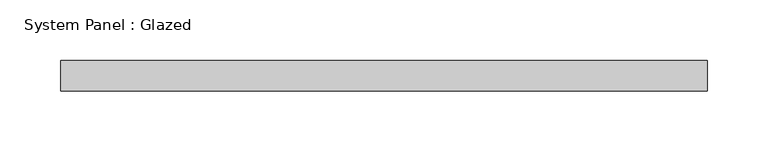
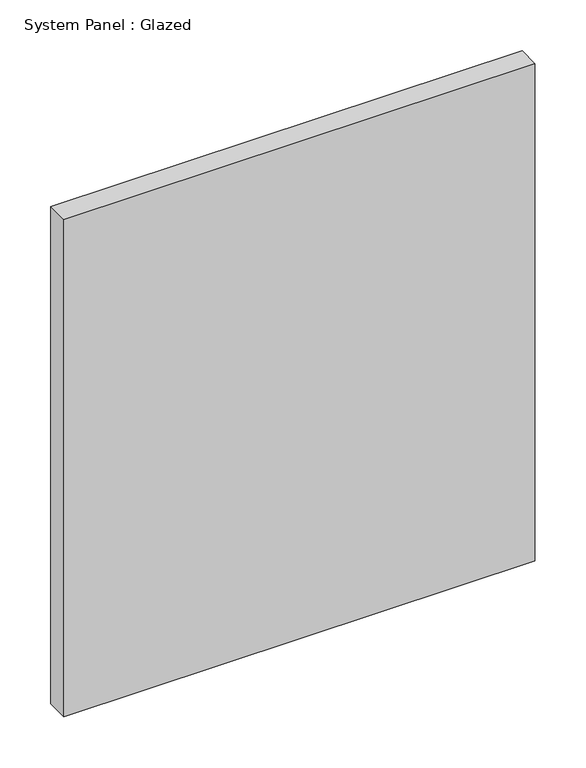
"""IFC4 building model written with IfcOpenShell, lengths in millimetres: plate geometry, System Panel : Glazed."""

from ifc_helpers import new_model, si_unit, origin, origin_with_axes, place, context, project, spatial, polyline, outline, extrude, source, transform, mapped, element, save


def system_panel_glazed_209ba7b6(model_context):
    return source(origin(), model_context, "Body", "SweptSolid", [
        extrude(outline(polyline([(266.7, 19.05), (-266.7, 19.05), (-266.7, 44.45), (266.7, 44.45), (266.7, 19.05)])), origin_with_axes(), (0.0, 0.0, 1.0), 595.2240338),
    ])


if __name__ == "__main__":
    model = new_model("IFC4")
    model_context = context("Model", 3, world=origin())
    ifc_project = project(units=[si_unit("LENGTHUNIT", "METRE", prefix="MILLI")], contexts=[model_context])
    site = spatial("IfcSite", under=ifc_project)
    building = spatial("IfcBuilding", under=site)
    placement = place(None, origin())
    system_panel_glazed_shape = system_panel_glazed_209ba7b6(model_context)
    element("IfcPlate", 1, ObjectType="System Panel : Glazed", at=placement, inside=building, context=model_context, shape_type="MappedRepresentation", body=[
        mapped(system_panel_glazed_shape, transform((0.0, 0.0, 0.0), x_axis=(1.0, 0.0, 0.0), y_axis=(0.0, 1.0, 0.0), z_axis=(0.0, 0.0, 1.0))),
    ])
    save(model, "model.ifc")

# Revit data of these elements
# Type "System Panel : Glazed"
#   Construction Type Id = "GSP4R"
#   Analytic Construction = "1/8 in Pilkington single glazing"
#   Visual Light Transmittance = 0.9
#   Solar Heat Gain Coefficient = 0.86
#   Heat Transfer Coefficient (U) = 1.18115 BTU/(h·ft²·°F)
#   Define Thermal Properties by = 1
# Element 1 (IfcPlate, "System Panel : Glazed")
#   Materials on its faces: "Glass"
# Materials
#   "Glass": class "Glass", colour RGB 0 128 192, transparency 0.75, Description = "Soda Lime Glass", Cost = 0
